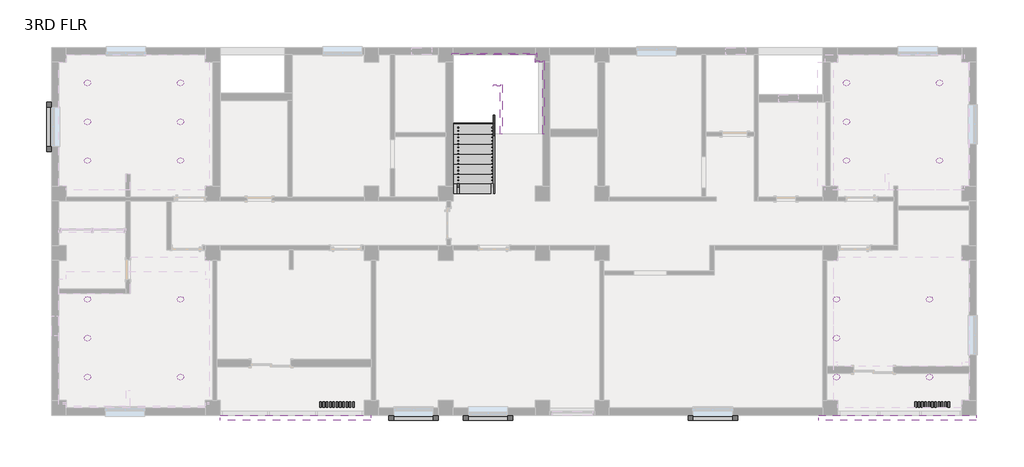
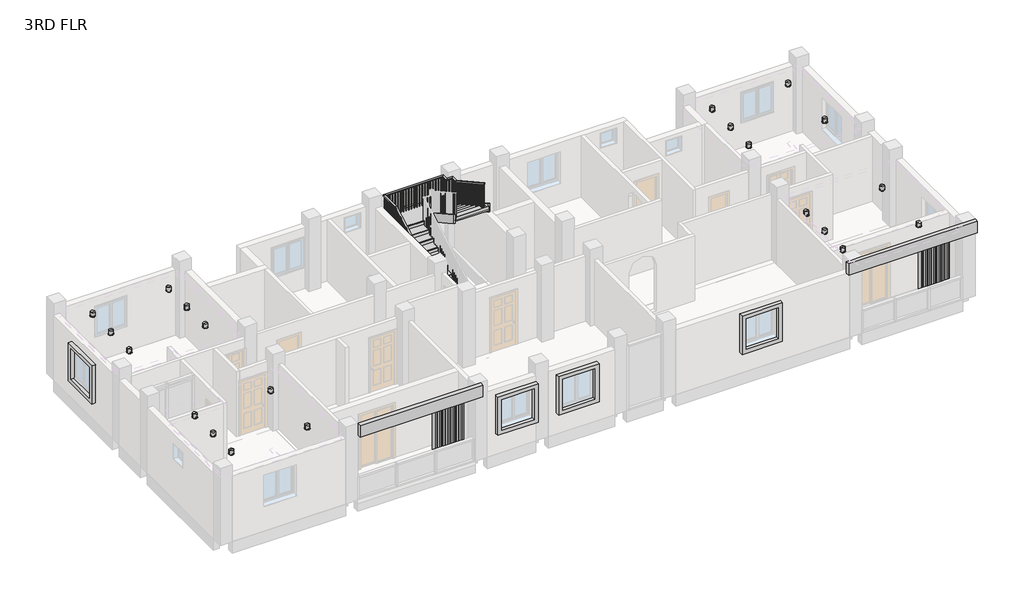
# One storey, part 5 of 5: 21 light fixtures, 8 members, 8 proxies, 1 railing, 1 stair flight.
# Revit data of these elements (continued)
# Element 27 (IfcLightFixture, "LIGHT_-_MODERN_PENDANT_14774 : Baffle") (continued)
#   Materials on its faces: "Metal - Paint Finish - Ivory,Glossy"
# Element 28 (IfcLightFixture, "LIGHT_-_MODERN_PENDANT_14774 : Baffle")
#   Mark = "57"
#   Wall Wash Reflector = none
#   Reflector = none
#   Fresnel Material = none
#   Phase Created = New Construction
#   Materials on its faces: "Metal - Paint Finish - Ivory,Glossy"
# Element 29 (IfcLightFixture, "LIGHT_-_MODERN_PENDANT_14774 : Baffle")
#   Mark = "58"
#   Wall Wash Reflector = none
#   Reflector = none
#   Fresnel Material = none
#   Phase Created = New Construction
#   Materials on its faces: "Metal - Paint Finish - Ivory,Glossy"
# Elements 30, 31, 32, 33, 34, 35, 36, 37 (IfcMember, "Stringer - 2\" Width")
#   Phase Created = New Construction
# Element 38 (IfcRailing, "Handrail - Rectangular")
#   Phase Created = New Construction
# Element 39 (IfcStairFlight, "2\" Tread 1\" Nosing 1/4\" Riser")
#   Phase Created = New Construction
# Materials
#   "Metal - Paint Finish - Ivory,Glossy": colour RGB 247 247 239, transparency 0
#   "WALL ACCENT 6\"": class "Generic", colour RGB 120 120 120, transparency 0, Cost = 0
#   "TEAK BROWN COLOUR": class "Generic", colour RGB 120 120 120, transparency 0, Cost = 0
